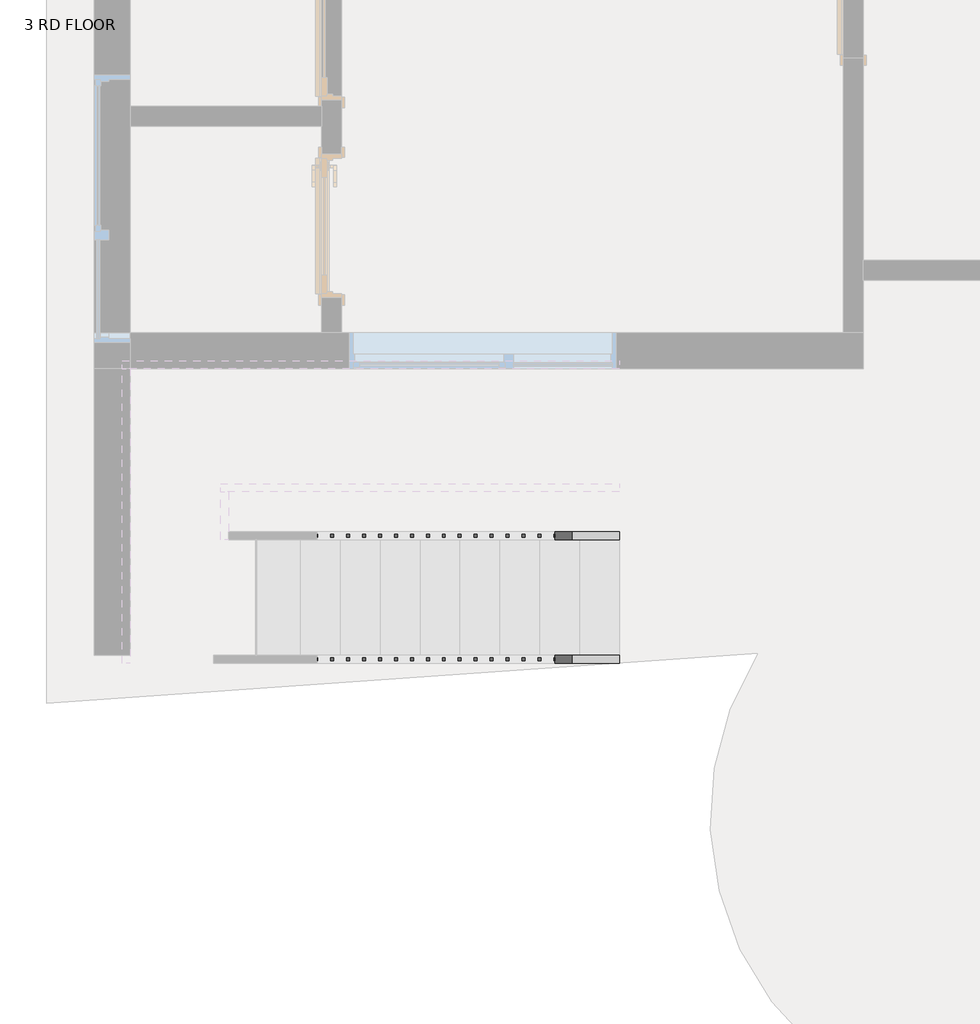
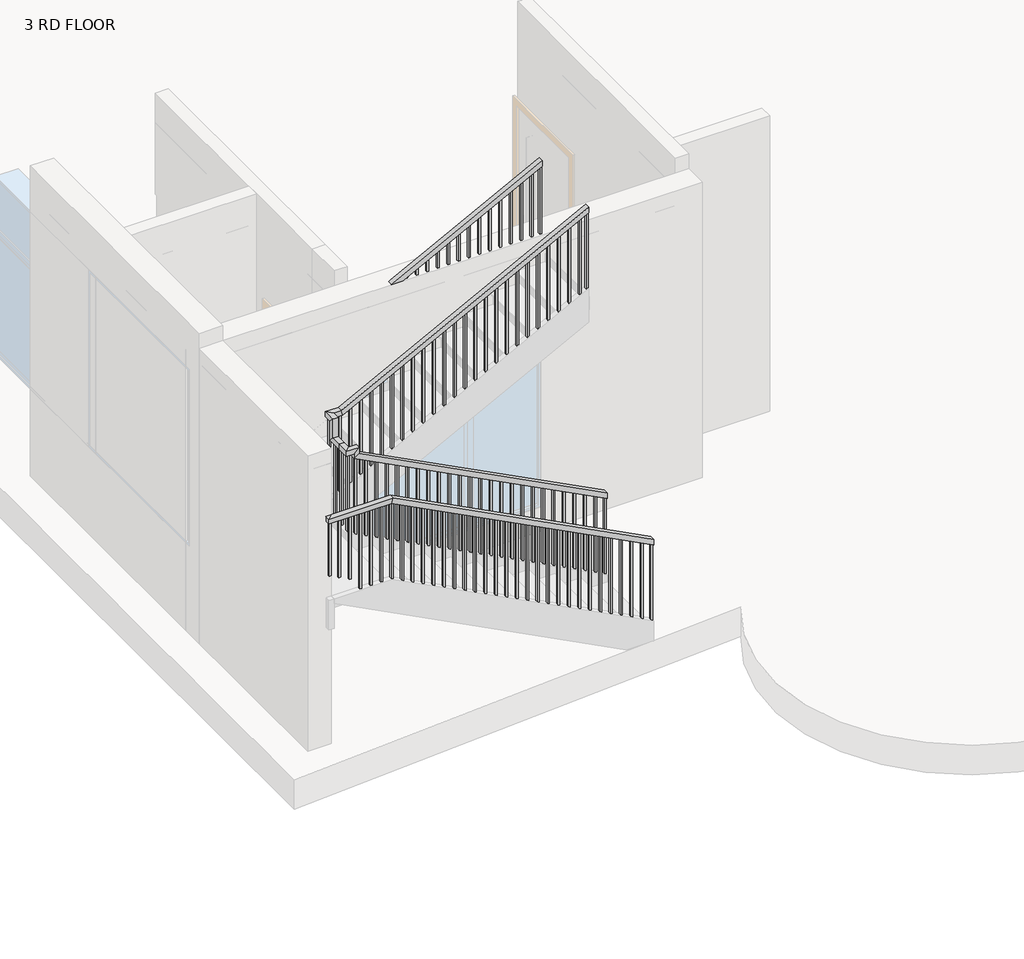
# One storey, part 4 of 5: 2 railings.
"""IFC4 building model written with IfcOpenShell, lengths in millimetres."""

from ifc_helpers import new_model, si_unit, frame, origin, place, context, project, spatial, polyline, outline, extrude, faceted_brep, element, save

model = new_model("IFC4")

# Units and contexts
model_context = context("Model", 3, world=origin())
ifc_project = project(units=[si_unit("LENGTHUNIT", "METRE", prefix="MILLI")], contexts=[model_context])

# Site, building, storey
site = spatial("IfcSite", under=ifc_project)
building = spatial("IfcBuilding", under=site)
storey = spatial("IfcBuildingStorey", under=building, Name="3 RD FLOOR", Elevation=9601.2)

# Railings
placement = place(None, origin())
element("IfcRailing", 1, ObjectType="Handrail - Rectangular", at=placement, inside=storey, context=model_context, shape_type="SolidModel", body=[
    faceted_brep([(-3117.2664982, -6914.3822004, 10647.2181818), (-3117.2664982, -6914.3822004, 10590.003028), (-3117.2664982, -6863.5822004, 10590.003028), (-3117.2664982, -6863.5822004, 10647.2181818), (-5530.2664982, -6914.3822004, 11897.5909091), (-5581.0664982, -6914.3822004, 11866.6993916), (-5581.0664982, -6863.5822004, 11866.6993916), (-5530.2664982, -6863.5822004, 11897.5909091), (-5657.2664982, -6787.3822004, 11912.6), (-5657.2664982, -6787.3822004, 11963.4), (-5657.2664982, -6685.7822004, 11963.4), (-5657.2664982, -6634.9822004, 11912.6), (-5606.4664982, -6787.3822004, 11912.6), (-5606.4664982, -6634.9822004, 11912.6), (-5606.4664982, -6787.3822004, 11963.4), (-5606.4664982, -6685.7822004, 11963.4), (-3117.2664982, -6558.7822004, 13411.2), (-3117.2664982, -6609.5822004, 13411.2), (-3117.2664982, -6609.5822004, 13353.9848461), (-3117.2664982, -6558.7822004, 13353.9848461), (-5517.8863767, -6558.7822004, 12110.0272727), (-5530.2664982, -6558.7822004, 12160.8272727), (-5517.8863767, -6609.5822004, 12110.0272727), (-5530.2664982, -6609.5822004, 12160.8272727), (-5530.2664982, -6914.3822004, 11963.4), (-5581.0664982, -6914.3822004, 11912.6), (-5581.0664982, -6863.5822004, 11912.6), (-5530.2664982, -6863.5822004, 11963.4), (-5657.2664982, -6914.3822004, 11963.4), (-5657.2664982, -6914.3822004, 11912.6), (-5606.4664982, -6863.5822004, 11912.6), (-5606.4664982, -6863.5822004, 11963.4), (-5657.2664982, -6685.7822004, 12160.8272727), (-5657.2664982, -6634.9822004, 12110.0272727), (-5606.4664982, -6634.9822004, 12110.0272727), (-5606.4664982, -6685.7822004, 12160.8272727), (-5657.2664982, -6558.7822004, 12160.8272727), (-5657.2664982, -6558.7822004, 12110.0272727), (-5606.4664982, -6609.5822004, 12110.0272727), (-5606.4664982, -6609.5822004, 12160.8272727)], [[[0, 1, 2, 3]], [[1, 0, 4, 5]], [[2, 1, 5, 6]], [[3, 2, 6, 7]], [[0, 3, 7, 4]], [[8, 9, 10, 11]], [[12, 8, 11, 13]], [[14, 12, 13, 15]], [[9, 14, 15, 10]], [[16, 17, 18, 19]], [[20, 21, 16, 19]], [[22, 20, 19, 18]], [[23, 22, 18, 17]], [[21, 23, 17, 16]], [[5, 4, 24, 25]], [[6, 5, 25, 26]], [[7, 6, 26, 27]], [[4, 7, 27, 24]], [[25, 24, 28, 29]], [[26, 25, 29, 30]], [[27, 26, 30, 31]], [[24, 27, 31, 28]], [[29, 28, 9, 8]], [[30, 29, 8, 12]], [[31, 30, 12, 14]], [[28, 31, 14, 9]], [[11, 10, 32, 33]], [[13, 11, 33, 34]], [[15, 13, 34, 35]], [[10, 15, 35, 32]], [[33, 32, 36, 37]], [[34, 33, 37, 38]], [[35, 34, 38, 39]], [[32, 35, 39, 36]], [[37, 36, 21, 20]], [[38, 37, 20, 22]], [[39, 38, 22, 23]], [[36, 39, 23, 21]]]),
    extrude(outline(polyline([(13319.4350734, -3183.9414982), (13309.5637098, -3202.9914982), (12525.2803899, -3202.9914982), (12535.1517536, -3183.9414982), (13319.4350734, -3183.9414982)])), frame((0.0, -6593.7072004, 0.0), z_axis=(0.0, 1.0, 0.0), x_axis=(0.0, 0.0, 1.0)), (0.0, 0.0, 1.0), 19.05),
    extrude(outline(polyline([(13266.7878007, -3285.5414982), (13256.916437, -3304.5914982), (12472.6331172, -3304.5914982), (12482.5044808, -3285.5414982), (13266.7878007, -3285.5414982)])), frame((0.0, -6593.7072004, 0.0), z_axis=(0.0, 1.0, 0.0), x_axis=(0.0, 0.0, 1.0)), (0.0, 0.0, 1.0), 19.05),
    extrude(outline(polyline([(13214.140528, -3387.1414982), (13204.2691643, -3406.1914982), (12419.9858445, -3406.1914982), (12429.8572081, -3387.1414982), (13214.140528, -3387.1414982)])), frame((0.0, -6593.7072004, 0.0), z_axis=(0.0, 1.0, 0.0), x_axis=(0.0, 0.0, 1.0)), (0.0, 0.0, 1.0), 19.05),
    extrude(outline(polyline([(13161.4932552, -3488.7414982), (13151.6218916, -3507.7914982), (12367.3385718, -3507.7914982), (12377.2099354, -3488.7414982), (13161.4932552, -3488.7414982)])), frame((0.0, -6593.7072004, 0.0), z_axis=(0.0, 1.0, 0.0), x_axis=(0.0, 0.0, 1.0)), (0.0, 0.0, 1.0), 19.05),
    extrude(outline(polyline([(13108.8459825, -3590.3414982), (13098.9746189, -3609.3914982), (12314.691299, -3609.3914982), (12324.5626627, -3590.3414982), (13108.8459825, -3590.3414982)])), frame((0.0, -6593.7072004, 0.0), z_axis=(0.0, 1.0, 0.0), x_axis=(0.0, 0.0, 1.0)), (0.0, 0.0, 1.0), 19.05),
    extrude(outline(polyline([(13056.1987098, -3691.9414982), (13046.3273461, -3710.9914982), (12262.0440263, -3710.9914982), (12271.9153899, -3691.9414982), (13056.1987098, -3691.9414982)])), frame((0.0, -6593.7072004, 0.0), z_axis=(0.0, 1.0, 0.0), x_axis=(0.0, 0.0, 1.0)), (0.0, 0.0, 1.0), 19.05),
    extrude(outline(polyline([(13003.551437, -3793.5414982), (12993.6800734, -3812.5914982), (12209.3967536, -3812.5914982), (12219.2681172, -3793.5414982), (13003.551437, -3793.5414982)])), frame((0.0, -6593.7072004, 0.0), z_axis=(0.0, 1.0, 0.0), x_axis=(0.0, 0.0, 1.0)), (0.0, 0.0, 1.0), 19.05),
    extrude(outline(polyline([(12950.9041643, -3895.1414982), (12941.0328007, -3914.1914982), (12156.7494808, -3914.1914982), (12166.6208445, -3895.1414982), (12950.9041643, -3895.1414982)])), frame((0.0, -6593.7072004, 0.0), z_axis=(0.0, 1.0, 0.0), x_axis=(0.0, 0.0, 1.0)), (0.0, 0.0, 1.0), 19.05),
    extrude(outline(polyline([(12898.2568916, -3996.7414982), (12888.385528, -4015.7914982), (12104.1022081, -4015.7914982), (12113.9735718, -3996.7414982), (12898.2568916, -3996.7414982)])), frame((0.0, -6593.7072004, 0.0), z_axis=(0.0, 1.0, 0.0), x_axis=(0.0, 0.0, 1.0)), (0.0, 0.0, 1.0), 19.05),
    extrude(outline(polyline([(12845.6096189, -4098.3414982), (12835.7382552, -4117.3914982), (12051.4549354, -4117.3914982), (12061.326299, -4098.3414982), (12845.6096189, -4098.3414982)])), frame((0.0, -6593.7072004, 0.0), z_axis=(0.0, 1.0, 0.0), x_axis=(0.0, 0.0, 1.0)), (0.0, 0.0, 1.0), 19.05),
    extrude(outline(polyline([(12792.9623461, -4199.9414982), (12783.0909825, -4218.9914982), (11998.8076627, -4218.9914982), (12008.6790263, -4199.9414982), (12792.9623461, -4199.9414982)])), frame((0.0, -6593.7072004, 0.0), z_axis=(0.0, 1.0, 0.0), x_axis=(0.0, 0.0, 1.0)), (0.0, 0.0, 1.0), 19.05),
    extrude(outline(polyline([(12740.3150734, -4301.5414982), (12730.4437098, -4320.5914982), (11946.1603899, -4320.5914982), (11956.0317536, -4301.5414982), (12740.3150734, -4301.5414982)])), frame((0.0, -6593.7072004, 0.0), z_axis=(0.0, 1.0, 0.0), x_axis=(0.0, 0.0, 1.0)), (0.0, 0.0, 1.0), 19.05),
    extrude(outline(polyline([(12687.6678007, -4403.1414982), (12677.796437, -4422.1914982), (11893.5131172, -4422.1914982), (11903.3844808, -4403.1414982), (12687.6678007, -4403.1414982)])), frame((0.0, -6593.7072004, 0.0), z_axis=(0.0, 1.0, 0.0), x_axis=(0.0, 0.0, 1.0)), (0.0, 0.0, 1.0), 19.05),
    extrude(outline(polyline([(12635.020528, -4504.7414982), (12625.1491643, -4523.7914982), (11840.8658445, -4523.7914982), (11850.7372081, -4504.7414982), (12635.020528, -4504.7414982)])), frame((0.0, -6593.7072004, 0.0), z_axis=(0.0, 1.0, 0.0), x_axis=(0.0, 0.0, 1.0)), (0.0, 0.0, 1.0), 19.05),
    extrude(outline(polyline([(12582.3732552, -4606.3414982), (12572.5018916, -4625.3914982), (11788.2185718, -4625.3914982), (11798.0899354, -4606.3414982), (12582.3732552, -4606.3414982)])), frame((0.0, -6593.7072004, 0.0), z_axis=(0.0, 1.0, 0.0), x_axis=(0.0, 0.0, 1.0)), (0.0, 0.0, 1.0), 19.05),
    extrude(outline(polyline([(12529.7259825, -4707.9414982), (12519.8546189, -4726.9914982), (11735.571299, -4726.9914982), (11745.4426627, -4707.9414982), (12529.7259825, -4707.9414982)])), frame((0.0, -6593.7072004, 0.0), z_axis=(0.0, 1.0, 0.0), x_axis=(0.0, 0.0, 1.0)), (0.0, 0.0, 1.0), 19.05),
    extrude(outline(polyline([(12477.0787098, -4809.5414982), (12467.2073461, -4828.5914982), (11682.9240263, -4828.5914982), (11692.7953899, -4809.5414982), (12477.0787098, -4809.5414982)])), frame((0.0, -6593.7072004, 0.0), z_axis=(0.0, 1.0, 0.0), x_axis=(0.0, 0.0, 1.0)), (0.0, 0.0, 1.0), 19.05),
    extrude(outline(polyline([(12424.431437, -4911.1414982), (12414.5600734, -4930.1914982), (11630.2767536, -4930.1914982), (11640.1481172, -4911.1414982), (12424.431437, -4911.1414982)])), frame((0.0, -6593.7072004, 0.0), z_axis=(0.0, 1.0, 0.0), x_axis=(0.0, 0.0, 1.0)), (0.0, 0.0, 1.0), 19.05),
    extrude(outline(polyline([(12371.7841643, -5012.7414982), (12361.9128007, -5031.7914982), (11577.6294808, -5031.7914982), (11587.5008445, -5012.7414982), (12371.7841643, -5012.7414982)])), frame((0.0, -6593.7072004, 0.0), z_axis=(0.0, 1.0, 0.0), x_axis=(0.0, 0.0, 1.0)), (0.0, 0.0, 1.0), 19.05),
    extrude(outline(polyline([(12319.1368916, -5114.3414982), (12309.265528, -5133.3914982), (11524.9822081, -5133.3914982), (11534.8535718, -5114.3414982), (12319.1368916, -5114.3414982)])), frame((0.0, -6593.7072004, 0.0), z_axis=(0.0, 1.0, 0.0), x_axis=(0.0, 0.0, 1.0)), (0.0, 0.0, 1.0), 19.05),
    extrude(outline(polyline([(12266.4896189, -5215.9414982), (12256.6182552, -5234.9914982), (11472.3349354, -5234.9914982), (11482.206299, -5215.9414982), (12266.4896189, -5215.9414982)])), frame((0.0, -6593.7072004, 0.0), z_axis=(0.0, 1.0, 0.0), x_axis=(0.0, 0.0, 1.0)), (0.0, 0.0, 1.0), 19.05),
    extrude(outline(polyline([(12213.8423461, -5317.5414982), (12203.9709825, -5336.5914982), (11419.6876627, -5336.5914982), (11429.5590263, -5317.5414982), (12213.8423461, -5317.5414982)])), frame((0.0, -6593.7072004, 0.0), z_axis=(0.0, 1.0, 0.0), x_axis=(0.0, 0.0, 1.0)), (0.0, 0.0, 1.0), 19.05),
    extrude(outline(polyline([(12161.1950734, -5419.1414982), (12151.3237098, -5438.1914982), (11367.0403899, -5438.1914982), (11376.9117536, -5419.1414982), (12161.1950734, -5419.1414982)])), frame((0.0, -6593.7072004, 0.0), z_axis=(0.0, 1.0, 0.0), x_axis=(0.0, 0.0, 1.0)), (0.0, 0.0, 1.0), 19.05),
    extrude(outline(polyline([(12108.5478007, -5520.7414982), (12098.676437, -5539.7914982), (11314.3931172, -5539.7914982), (11324.2644808, -5520.7414982), (12108.5478007, -5520.7414982)])), frame((0.0, -6593.7072004, 0.0), z_axis=(0.0, 1.0, 0.0), x_axis=(0.0, 0.0, 1.0)), (0.0, 0.0, 1.0), 19.05),
    extrude(outline(polyline([(-5622.3414982, -6695.3072004), (-5641.3914982, -6695.3072004), (-5641.3914982, -6676.2572004), (-5622.3414982, -6676.2572004), (-5622.3414982, -6695.3072004)])), frame((0.0, 0.0, 11125.2), z_axis=(0.0, 0.0, 1.0), x_axis=(1.0, 0.0, 0.0)), (0.0, 0.0, 1.0), 787.4),
    extrude(outline(polyline([(-5622.3414982, -6796.9072004), (-5641.3914982, -6796.9072004), (-5641.3914982, -6777.8572004), (-5622.3414982, -6777.8572004), (-5622.3414982, -6796.9072004)])), frame((0.0, 0.0, 11125.2), z_axis=(0.0, 0.0, 1.0), x_axis=(1.0, 0.0, 0.0)), (0.0, 0.0, 1.0), 787.4),
    extrude(outline(polyline([(11912.6, -5546.1414982), (11912.6, -5565.1914982), (11074.1899354, -5565.1914982), (11064.3185718, -5546.1414982), (11912.6, -5546.1414982)])), frame((0.0, -6898.5072004, 0.0), z_axis=(0.0, 1.0, 0.0), x_axis=(0.0, 0.0, 1.0)), (0.0, 0.0, 1.0), 19.05),
    extrude(outline(polyline([(11795.9546189, -5444.5414982), (11805.8259825, -5463.5914982), (11021.5426627, -5463.5914982), (11011.671299, -5444.5414982), (11795.9546189, -5444.5414982)])), frame((0.0, -6898.5072004, 0.0), z_axis=(0.0, 1.0, 0.0), x_axis=(0.0, 0.0, 1.0)), (0.0, 0.0, 1.0), 19.05),
    extrude(outline(polyline([(11743.3073461, -5342.9414982), (11753.1787098, -5361.9914982), (10968.8953899, -5361.9914982), (10959.0240263, -5342.9414982), (11743.3073461, -5342.9414982)])), frame((0.0, -6898.5072004, 0.0), z_axis=(0.0, 1.0, 0.0), x_axis=(0.0, 0.0, 1.0)), (0.0, 0.0, 1.0), 19.05),
    extrude(outline(polyline([(11690.6600734, -5241.3414982), (11700.531437, -5260.3914982), (10916.2481172, -5260.3914982), (10906.3767536, -5241.3414982), (11690.6600734, -5241.3414982)])), frame((0.0, -6898.5072004, 0.0), z_axis=(0.0, 1.0, 0.0), x_axis=(0.0, 0.0, 1.0)), (0.0, 0.0, 1.0), 19.05),
    extrude(outline(polyline([(11638.0128007, -5139.7414982), (11647.8841643, -5158.7914982), (10863.6008445, -5158.7914982), (10853.7294808, -5139.7414982), (11638.0128007, -5139.7414982)])), frame((0.0, -6898.5072004, 0.0), z_axis=(0.0, 1.0, 0.0), x_axis=(0.0, 0.0, 1.0)), (0.0, 0.0, 1.0), 19.05),
    extrude(outline(polyline([(11585.365528, -5038.1414982), (11595.2368916, -5057.1914982), (10810.9535718, -5057.1914982), (10801.0822081, -5038.1414982), (11585.365528, -5038.1414982)])), frame((0.0, -6898.5072004, 0.0), z_axis=(0.0, 1.0, 0.0), x_axis=(0.0, 0.0, 1.0)), (0.0, 0.0, 1.0), 19.05),
    extrude(outline(polyline([(11532.7182552, -4936.5414982), (11542.5896189, -4955.5914982), (10758.306299, -4955.5914982), (10748.4349354, -4936.5414982), (11532.7182552, -4936.5414982)])), frame((0.0, -6898.5072004, 0.0), z_axis=(0.0, 1.0, 0.0), x_axis=(0.0, 0.0, 1.0)), (0.0, 0.0, 1.0), 19.05),
    extrude(outline(polyline([(11480.0709825, -4834.9414982), (11489.9423461, -4853.9914982), (10705.6590263, -4853.9914982), (10695.7876627, -4834.9414982), (11480.0709825, -4834.9414982)])), frame((0.0, -6898.5072004, 0.0), z_axis=(0.0, 1.0, 0.0), x_axis=(0.0, 0.0, 1.0)), (0.0, 0.0, 1.0), 19.05),
    extrude(outline(polyline([(11427.4237098, -4733.3414982), (11437.2950734, -4752.3914982), (10653.0117536, -4752.3914982), (10643.1403899, -4733.3414982), (11427.4237098, -4733.3414982)])), frame((0.0, -6898.5072004, 0.0), z_axis=(0.0, 1.0, 0.0), x_axis=(0.0, 0.0, 1.0)), (0.0, 0.0, 1.0), 19.05),
    extrude(outline(polyline([(11374.776437, -4631.7414982), (11384.6478007, -4650.7914982), (10600.3644808, -4650.7914982), (10590.4931172, -4631.7414982), (11374.776437, -4631.7414982)])), frame((0.0, -6898.5072004, 0.0), z_axis=(0.0, 1.0, 0.0), x_axis=(0.0, 0.0, 1.0)), (0.0, 0.0, 1.0), 19.05),
    extrude(outline(polyline([(11322.1291643, -4530.1414982), (11332.000528, -4549.1914982), (10547.7172081, -4549.1914982), (10537.8458445, -4530.1414982), (11322.1291643, -4530.1414982)])), frame((0.0, -6898.5072004, 0.0), z_axis=(0.0, 1.0, 0.0), x_axis=(0.0, 0.0, 1.0)), (0.0, 0.0, 1.0), 19.05),
    extrude(outline(polyline([(11269.4818916, -4428.5414982), (11279.3532552, -4447.5914982), (10495.0699354, -4447.5914982), (10485.1985718, -4428.5414982), (11269.4818916, -4428.5414982)])), frame((0.0, -6898.5072004, 0.0), z_axis=(0.0, 1.0, 0.0), x_axis=(0.0, 0.0, 1.0)), (0.0, 0.0, 1.0), 19.05),
    extrude(outline(polyline([(11216.8346189, -4326.9414982), (11226.7059825, -4345.9914982), (10442.4226627, -4345.9914982), (10432.551299, -4326.9414982), (11216.8346189, -4326.9414982)])), frame((0.0, -6898.5072004, 0.0), z_axis=(0.0, 1.0, 0.0), x_axis=(0.0, 0.0, 1.0)), (0.0, 0.0, 1.0), 19.05),
    extrude(outline(polyline([(11164.1873461, -4225.3414982), (11174.0587098, -4244.3914982), (10389.7753899, -4244.3914982), (10379.9040263, -4225.3414982), (11164.1873461, -4225.3414982)])), frame((0.0, -6898.5072004, 0.0), z_axis=(0.0, 1.0, 0.0), x_axis=(0.0, 0.0, 1.0)), (0.0, 0.0, 1.0), 19.05),
    extrude(outline(polyline([(11111.5400734, -4123.7414982), (11121.411437, -4142.7914982), (10337.1281172, -4142.7914982), (10327.2567536, -4123.7414982), (11111.5400734, -4123.7414982)])), frame((0.0, -6898.5072004, 0.0), z_axis=(0.0, 1.0, 0.0), x_axis=(0.0, 0.0, 1.0)), (0.0, 0.0, 1.0), 19.05),
    extrude(outline(polyline([(11058.8928007, -4022.1414982), (11068.7641643, -4041.1914982), (10284.4808445, -4041.1914982), (10274.6094808, -4022.1414982), (11058.8928007, -4022.1414982)])), frame((0.0, -6898.5072004, 0.0), z_axis=(0.0, 1.0, 0.0), x_axis=(0.0, 0.0, 1.0)), (0.0, 0.0, 1.0), 19.05),
    extrude(outline(polyline([(11006.245528, -3920.5414982), (11016.1168916, -3939.5914982), (10231.8335718, -3939.5914982), (10221.9622081, -3920.5414982), (11006.245528, -3920.5414982)])), frame((0.0, -6898.5072004, 0.0), z_axis=(0.0, 1.0, 0.0), x_axis=(0.0, 0.0, 1.0)), (0.0, 0.0, 1.0), 19.05),
    extrude(outline(polyline([(10953.5982552, -3818.9414982), (10963.4696189, -3837.9914982), (10179.186299, -3837.9914982), (10169.3149354, -3818.9414982), (10953.5982552, -3818.9414982)])), frame((0.0, -6898.5072004, 0.0), z_axis=(0.0, 1.0, 0.0), x_axis=(0.0, 0.0, 1.0)), (0.0, 0.0, 1.0), 19.05),
    extrude(outline(polyline([(10900.9509825, -3717.3414982), (10910.8223461, -3736.3914982), (10126.5390263, -3736.3914982), (10116.6676627, -3717.3414982), (10900.9509825, -3717.3414982)])), frame((0.0, -6898.5072004, 0.0), z_axis=(0.0, 1.0, 0.0), x_axis=(0.0, 0.0, 1.0)), (0.0, 0.0, 1.0), 19.05),
    extrude(outline(polyline([(10848.3037098, -3615.7414982), (10858.1750734, -3634.7914982), (10073.8917536, -3634.7914982), (10064.0203899, -3615.7414982), (10848.3037098, -3615.7414982)])), frame((0.0, -6898.5072004, 0.0), z_axis=(0.0, 1.0, 0.0), x_axis=(0.0, 0.0, 1.0)), (0.0, 0.0, 1.0), 19.05),
    extrude(outline(polyline([(10795.656437, -3514.1414982), (10805.5278007, -3533.1914982), (10021.2444808, -3533.1914982), (10011.3731172, -3514.1414982), (10795.656437, -3514.1414982)])), frame((0.0, -6898.5072004, 0.0), z_axis=(0.0, 1.0, 0.0), x_axis=(0.0, 0.0, 1.0)), (0.0, 0.0, 1.0), 19.05),
    extrude(outline(polyline([(10743.0091643, -3412.5414982), (10752.880528, -3431.5914982), (9968.5972081, -3431.5914982), (9958.7258445, -3412.5414982), (10743.0091643, -3412.5414982)])), frame((0.0, -6898.5072004, 0.0), z_axis=(0.0, 1.0, 0.0), x_axis=(0.0, 0.0, 1.0)), (0.0, 0.0, 1.0), 19.05),
    extrude(outline(polyline([(10690.3618916, -3310.9414982), (10700.2332552, -3329.9914982), (9915.9499354, -3329.9914982), (9906.0785718, -3310.9414982), (10690.3618916, -3310.9414982)])), frame((0.0, -6898.5072004, 0.0), z_axis=(0.0, 1.0, 0.0), x_axis=(0.0, 0.0, 1.0)), (0.0, 0.0, 1.0), 19.05),
    extrude(outline(polyline([(10637.7146189, -3209.3414982), (10647.5859825, -3228.3914982), (9863.3026627, -3228.3914982), (9853.431299, -3209.3414982), (10637.7146189, -3209.3414982)])), frame((0.0, -6898.5072004, 0.0), z_axis=(0.0, 1.0, 0.0), x_axis=(0.0, 0.0, 1.0)), (0.0, 0.0, 1.0), 19.05),
    extrude(outline(polyline([(-6593.7072004, 12110.0272727), (-6574.6572004, 12110.0272727), (-6574.6572004, 11271.6172081), (-6593.7072004, 11261.7458445), (-6593.7072004, 12110.0272727)])), frame((-5641.3914982, 0.0, 0.0), z_axis=(1.0, 0.0, 0.0), x_axis=(0.0, 1.0, 0.0)), (0.0, 0.0, 1.0), 19.05),
    extrude(outline(polyline([(-5622.3414982, -6879.4572004), (-5622.3414982, -6898.5072004), (-5641.3914982, -6898.5072004), (-5641.3914982, -6879.4572004), (-5622.3414982, -6879.4572004)])), frame((0.0, 0.0, 11125.2), z_axis=(0.0, 0.0, 1.0), x_axis=(1.0, 0.0, 0.0)), (0.0, 0.0, 1.0), 787.4),
    extrude(outline(polyline([(13353.9848461, -3117.2664982), (13344.1134825, -3136.3164982), (12559.8301627, -3136.3164982), (12569.7015263, -3117.2664982), (13353.9848461, -3117.2664982)])), frame((0.0, -6593.7072004, 0.0), z_axis=(0.0, 1.0, 0.0), x_axis=(0.0, 0.0, 1.0)), (0.0, 0.0, 1.0), 19.05),
    extrude(outline(polyline([(10590.003028, -3117.2664982), (10599.8743916, -3136.3164982), (9815.5910718, -3136.3164982), (9805.7197081, -3117.2664982), (10590.003028, -3117.2664982)])), frame((0.0, -6898.5072004, 0.0), z_axis=(0.0, 1.0, 0.0), x_axis=(0.0, 0.0, 1.0)), (0.0, 0.0, 1.0), 19.05),
])
element("IfcRailing", 2, ObjectType="Handrail - Rectangular", at=placement, inside=storey, context=model_context, shape_type="SolidModel", body=[
    faceted_brep([(-3117.2664982, -7701.7822004, 10647.2181818), (-3117.2664982, -7701.7822004, 10590.003028), (-3117.2664982, -7650.9822004, 10590.003028), (-3117.2664982, -7650.9822004, 10647.2181818), (-5657.2664982, -7701.7822004, 11963.4), (-5669.6466197, -7701.7822004, 11912.6), (-5669.6466197, -7650.9822004, 11912.6), (-5657.2664982, -7650.9822004, 11963.4), (-6283.3131972, -7701.7822004, 11912.6), (-6283.3131972, -7701.7822004, 11963.4), (-6283.3131972, -5773.9082131, 11963.4), (-6283.3131972, -5773.9082131, 11912.6), (-6232.5131972, -7650.9822004, 11912.6), (-6232.5131972, -5824.7082131, 11912.6), (-6232.5131972, -7650.9822004, 11963.4), (-6232.5131972, -5824.7082131, 11963.4), (-5911.2664982, -5773.9082131, 11963.4), (-5898.8863767, -5773.9082131, 11912.6), (-5898.8863767, -5824.7082131, 11912.6), (-5911.2664982, -5824.7082131, 11963.4), (-3117.2664982, -5773.9082131, 13411.2), (-3117.2664982, -5824.7082131, 13411.2), (-3117.2664982, -5824.7082131, 13353.9848461), (-3117.2664982, -5773.9082131, 13353.9848461)], [[[0, 1, 2, 3]], [[1, 0, 4, 5]], [[2, 1, 5, 6]], [[3, 2, 6, 7]], [[0, 3, 7, 4]], [[8, 9, 10, 11]], [[12, 8, 11, 13]], [[14, 12, 13, 15]], [[9, 14, 15, 10]], [[11, 10, 16, 17]], [[13, 11, 17, 18]], [[15, 13, 18, 19]], [[10, 15, 19, 16]], [[5, 4, 9, 8]], [[6, 5, 8, 12]], [[7, 6, 12, 14]], [[4, 7, 14, 9]], [[20, 21, 22, 23]], [[17, 16, 20, 23]], [[18, 17, 23, 22]], [[19, 18, 22, 21]], [[16, 19, 21, 20]]]),
    extrude(outline(polyline([(13301.0413294, -3219.4381972), (12516.7580095, -3219.4381972), (12526.6293732, -3200.3881972), (13310.912693, -3200.3881972), (13301.0413294, -3219.4381972)])), frame((0.0, -5808.8332131, 0.0), z_axis=(0.0, 1.0, 0.0), x_axis=(0.0, 0.0, 1.0)), (0.0, 0.0, 1.0), 19.05),
    extrude(outline(polyline([(13248.3940566, -3321.0381972), (12464.1107368, -3321.0381972), (12473.9821004, -3301.9881972), (13258.2654203, -3301.9881972), (13248.3940566, -3321.0381972)])), frame((0.0, -5808.8332131, 0.0), z_axis=(0.0, 1.0, 0.0), x_axis=(0.0, 0.0, 1.0)), (0.0, 0.0, 1.0), 19.05),
    extrude(outline(polyline([(13195.7467839, -3422.6381972), (12411.4634641, -3422.6381972), (12421.3348277, -3403.5881972), (13205.6181476, -3403.5881972), (13195.7467839, -3422.6381972)])), frame((0.0, -5808.8332131, 0.0), z_axis=(0.0, 1.0, 0.0), x_axis=(0.0, 0.0, 1.0)), (0.0, 0.0, 1.0), 19.05),
    extrude(outline(polyline([(13143.0995112, -3524.2381972), (12358.8161913, -3524.2381972), (12368.687555, -3505.1881972), (13152.9708748, -3505.1881972), (13143.0995112, -3524.2381972)])), frame((0.0, -5808.8332131, 0.0), z_axis=(0.0, 1.0, 0.0), x_axis=(0.0, 0.0, 1.0)), (0.0, 0.0, 1.0), 19.05),
    extrude(outline(polyline([(13090.4522385, -3625.8381972), (12306.1689186, -3625.8381972), (12316.0402823, -3606.7881972), (13100.3236021, -3606.7881972), (13090.4522385, -3625.8381972)])), frame((0.0, -5808.8332131, 0.0), z_axis=(0.0, 1.0, 0.0), x_axis=(0.0, 0.0, 1.0)), (0.0, 0.0, 1.0), 19.05),
    extrude(outline(polyline([(13037.8049657, -3727.4381972), (12253.5216459, -3727.4381972), (12263.3930095, -3708.3881972), (13047.6763294, -3708.3881972), (13037.8049657, -3727.4381972)])), frame((0.0, -5808.8332131, 0.0), z_axis=(0.0, 1.0, 0.0), x_axis=(0.0, 0.0, 1.0)), (0.0, 0.0, 1.0), 19.05),
    extrude(outline(polyline([(12985.157693, -3829.0381972), (12200.8743732, -3829.0381972), (12210.7457368, -3809.9881972), (12995.0290566, -3809.9881972), (12985.157693, -3829.0381972)])), frame((0.0, -5808.8332131, 0.0), z_axis=(0.0, 1.0, 0.0), x_axis=(0.0, 0.0, 1.0)), (0.0, 0.0, 1.0), 19.05),
    extrude(outline(polyline([(12932.5104203, -3930.6381972), (12148.2271004, -3930.6381972), (12158.0984641, -3911.5881972), (12942.3817839, -3911.5881972), (12932.5104203, -3930.6381972)])), frame((0.0, -5808.8332131, 0.0), z_axis=(0.0, 1.0, 0.0), x_axis=(0.0, 0.0, 1.0)), (0.0, 0.0, 1.0), 19.05),
    extrude(outline(polyline([(12879.8631476, -4032.2381972), (12095.5798277, -4032.2381972), (12105.4511913, -4013.1881972), (12889.7345112, -4013.1881972), (12879.8631476, -4032.2381972)])), frame((0.0, -5808.8332131, 0.0), z_axis=(0.0, 1.0, 0.0), x_axis=(0.0, 0.0, 1.0)), (0.0, 0.0, 1.0), 19.05),
    extrude(outline(polyline([(12827.2158748, -4133.8381972), (12042.932555, -4133.8381972), (12052.8039186, -4114.7881972), (12837.0872385, -4114.7881972), (12827.2158748, -4133.8381972)])), frame((0.0, -5808.8332131, 0.0), z_axis=(0.0, 1.0, 0.0), x_axis=(0.0, 0.0, 1.0)), (0.0, 0.0, 1.0), 19.05),
    extrude(outline(polyline([(12774.5686021, -4235.4381972), (11990.2852823, -4235.4381972), (12000.1566459, -4216.3881972), (12784.4399657, -4216.3881972), (12774.5686021, -4235.4381972)])), frame((0.0, -5808.8332131, 0.0), z_axis=(0.0, 1.0, 0.0), x_axis=(0.0, 0.0, 1.0)), (0.0, 0.0, 1.0), 19.05),
    extrude(outline(polyline([(12721.9213294, -4337.0381972), (11937.6380095, -4337.0381972), (11947.5093732, -4317.9881972), (12731.792693, -4317.9881972), (12721.9213294, -4337.0381972)])), frame((0.0, -5808.8332131, 0.0), z_axis=(0.0, 1.0, 0.0), x_axis=(0.0, 0.0, 1.0)), (0.0, 0.0, 1.0), 19.05),
    extrude(outline(polyline([(12669.2740566, -4438.6381972), (11884.9907368, -4438.6381972), (11894.8621004, -4419.5881972), (12679.1454203, -4419.5881972), (12669.2740566, -4438.6381972)])), frame((0.0, -5808.8332131, 0.0), z_axis=(0.0, 1.0, 0.0), x_axis=(0.0, 0.0, 1.0)), (0.0, 0.0, 1.0), 19.05),
    extrude(outline(polyline([(12616.6267839, -4540.2381972), (11832.3434641, -4540.2381972), (11842.2148277, -4521.1881972), (12626.4981476, -4521.1881972), (12616.6267839, -4540.2381972)])), frame((0.0, -5808.8332131, 0.0), z_axis=(0.0, 1.0, 0.0), x_axis=(0.0, 0.0, 1.0)), (0.0, 0.0, 1.0), 19.05),
    extrude(outline(polyline([(12563.9795112, -4641.8381972), (11779.6961913, -4641.8381972), (11789.567555, -4622.7881972), (12573.8508748, -4622.7881972), (12563.9795112, -4641.8381972)])), frame((0.0, -5808.8332131, 0.0), z_axis=(0.0, 1.0, 0.0), x_axis=(0.0, 0.0, 1.0)), (0.0, 0.0, 1.0), 19.05),
    extrude(outline(polyline([(12511.3322385, -4743.4381972), (11727.0489186, -4743.4381972), (11736.9202823, -4724.3881972), (12521.2036021, -4724.3881972), (12511.3322385, -4743.4381972)])), frame((0.0, -5808.8332131, 0.0), z_axis=(0.0, 1.0, 0.0), x_axis=(0.0, 0.0, 1.0)), (0.0, 0.0, 1.0), 19.05),
    extrude(outline(polyline([(12458.6849657, -4845.0381972), (11674.4016459, -4845.0381972), (11684.2730095, -4825.9881972), (12468.5563294, -4825.9881972), (12458.6849657, -4845.0381972)])), frame((0.0, -5808.8332131, 0.0), z_axis=(0.0, 1.0, 0.0), x_axis=(0.0, 0.0, 1.0)), (0.0, 0.0, 1.0), 19.05),
    extrude(outline(polyline([(12406.037693, -4946.6381972), (11621.7543732, -4946.6381972), (11631.6257368, -4927.5881972), (12415.9090566, -4927.5881972), (12406.037693, -4946.6381972)])), frame((0.0, -5808.8332131, 0.0), z_axis=(0.0, 1.0, 0.0), x_axis=(0.0, 0.0, 1.0)), (0.0, 0.0, 1.0), 19.05),
    extrude(outline(polyline([(12353.3904203, -5048.2381972), (11569.1071004, -5048.2381972), (11578.9784641, -5029.1881972), (12363.2617839, -5029.1881972), (12353.3904203, -5048.2381972)])), frame((0.0, -5808.8332131, 0.0), z_axis=(0.0, 1.0, 0.0), x_axis=(0.0, 0.0, 1.0)), (0.0, 0.0, 1.0), 19.05),
    extrude(outline(polyline([(12300.7431476, -5149.8381972), (11516.4598277, -5149.8381972), (11526.3311913, -5130.7881972), (12310.6145112, -5130.7881972), (12300.7431476, -5149.8381972)])), frame((0.0, -5808.8332131, 0.0), z_axis=(0.0, 1.0, 0.0), x_axis=(0.0, 0.0, 1.0)), (0.0, 0.0, 1.0), 19.05),
    extrude(outline(polyline([(12248.0958748, -5251.4381972), (11463.812555, -5251.4381972), (11473.6839186, -5232.3881972), (12257.9672385, -5232.3881972), (12248.0958748, -5251.4381972)])), frame((0.0, -5808.8332131, 0.0), z_axis=(0.0, 1.0, 0.0), x_axis=(0.0, 0.0, 1.0)), (0.0, 0.0, 1.0), 19.05),
    extrude(outline(polyline([(12195.4486021, -5353.0381972), (11411.1652823, -5353.0381972), (11421.0366459, -5333.9881972), (12205.3199657, -5333.9881972), (12195.4486021, -5353.0381972)])), frame((0.0, -5808.8332131, 0.0), z_axis=(0.0, 1.0, 0.0), x_axis=(0.0, 0.0, 1.0)), (0.0, 0.0, 1.0), 19.05),
    extrude(outline(polyline([(12142.8013294, -5454.6381972), (11358.5180095, -5454.6381972), (11368.3893732, -5435.5881972), (12152.672693, -5435.5881972), (12142.8013294, -5454.6381972)])), frame((0.0, -5808.8332131, 0.0), z_axis=(0.0, 1.0, 0.0), x_axis=(0.0, 0.0, 1.0)), (0.0, 0.0, 1.0), 19.05),
    extrude(outline(polyline([(12090.1540566, -5556.2381972), (11305.8707368, -5556.2381972), (11315.7421004, -5537.1881972), (12100.0254203, -5537.1881972), (12090.1540566, -5556.2381972)])), frame((0.0, -5808.8332131, 0.0), z_axis=(0.0, 1.0, 0.0), x_axis=(0.0, 0.0, 1.0)), (0.0, 0.0, 1.0), 19.05),
    extrude(outline(polyline([(12037.5067839, -5657.8381972), (11253.2234641, -5657.8381972), (11263.0948277, -5638.7881972), (12047.3781476, -5638.7881972), (12037.5067839, -5657.8381972)])), frame((0.0, -5808.8332131, 0.0), z_axis=(0.0, 1.0, 0.0), x_axis=(0.0, 0.0, 1.0)), (0.0, 0.0, 1.0), 19.05),
    extrude(outline(polyline([(11984.8595112, -5759.4381972), (11200.5761913, -5759.4381972), (11210.447555, -5740.3881972), (11994.7308748, -5740.3881972), (11984.8595112, -5759.4381972)])), frame((0.0, -5808.8332131, 0.0), z_axis=(0.0, 1.0, 0.0), x_axis=(0.0, 0.0, 1.0)), (0.0, 0.0, 1.0), 19.05),
    extrude(outline(polyline([(11932.2122385, -5861.0381972), (11147.9289186, -5861.0381972), (11157.8002823, -5841.9881972), (11942.0836021, -5841.9881972), (11932.2122385, -5861.0381972)])), frame((0.0, -5808.8332131, 0.0), z_axis=(0.0, 1.0, 0.0), x_axis=(0.0, 0.0, 1.0)), (0.0, 0.0, 1.0), 19.05),
    extrude(outline(polyline([(11912.6, -5962.6381972), (11095.2816459, -5962.6381972), (11105.1530095, -5943.5881972), (11912.6, -5943.5881972), (11912.6, -5962.6381972)])), frame((0.0, -5808.8332131, 0.0), z_axis=(0.0, 1.0, 0.0), x_axis=(0.0, 0.0, 1.0)), (0.0, 0.0, 1.0), 19.05),
    extrude(outline(polyline([(11912.6, -6064.2381972), (11042.6343732, -6064.2381972), (11052.5057368, -6045.1881972), (11912.6, -6045.1881972), (11912.6, -6064.2381972)])), frame((0.0, -5808.8332131, 0.0), z_axis=(0.0, 1.0, 0.0), x_axis=(0.0, 0.0, 1.0)), (0.0, 0.0, 1.0), 19.05),
    extrude(outline(polyline([(11912.6, -6165.8381972), (10989.9871004, -6165.8381972), (10999.8584641, -6146.7881972), (11912.6, -6146.7881972), (11912.6, -6165.8381972)])), frame((0.0, -5808.8332131, 0.0), z_axis=(0.0, 1.0, 0.0), x_axis=(0.0, 0.0, 1.0)), (0.0, 0.0, 1.0), 19.05),
    extrude(outline(polyline([(-6267.4381972, -5857.1072004), (-6267.4381972, -5838.0572004), (-6248.3881972, -5838.0572004), (-6248.3881972, -5857.1072004), (-6267.4381972, -5857.1072004)])), frame((0.0, 0.0, 11125.2), z_axis=(0.0, 0.0, 1.0), x_axis=(1.0, 0.0, 0.0)), (0.0, 0.0, 1.0), 787.4),
    extrude(outline(polyline([(-6267.4381972, -5958.7072004), (-6267.4381972, -5939.6572004), (-6248.3881972, -5939.6572004), (-6248.3881972, -5958.7072004), (-6267.4381972, -5958.7072004)])), frame((0.0, 0.0, 11125.2), z_axis=(0.0, 0.0, 1.0), x_axis=(1.0, 0.0, 0.0)), (0.0, 0.0, 1.0), 787.4),
    extrude(outline(polyline([(-6267.4381972, -6060.3072004), (-6267.4381972, -6041.2572004), (-6248.3881972, -6041.2572004), (-6248.3881972, -6060.3072004), (-6267.4381972, -6060.3072004)])), frame((0.0, 0.0, 11125.2), z_axis=(0.0, 0.0, 1.0), x_axis=(1.0, 0.0, 0.0)), (0.0, 0.0, 1.0), 787.4),
    extrude(outline(polyline([(-6267.4381972, -6161.9072004), (-6267.4381972, -6142.8572004), (-6248.3881972, -6142.8572004), (-6248.3881972, -6161.9072004), (-6267.4381972, -6161.9072004)])), frame((0.0, 0.0, 11125.2), z_axis=(0.0, 0.0, 1.0), x_axis=(1.0, 0.0, 0.0)), (0.0, 0.0, 1.0), 787.4),
    extrude(outline(polyline([(-6267.4381972, -6263.5072004), (-6267.4381972, -6244.4572004), (-6248.3881972, -6244.4572004), (-6248.3881972, -6263.5072004), (-6267.4381972, -6263.5072004)])), frame((0.0, 0.0, 11125.2), z_axis=(0.0, 0.0, 1.0), x_axis=(1.0, 0.0, 0.0)), (0.0, 0.0, 1.0), 787.4),
    extrude(outline(polyline([(-6267.4381972, -6365.1072004), (-6267.4381972, -6346.0572004), (-6248.3881972, -6346.0572004), (-6248.3881972, -6365.1072004), (-6267.4381972, -6365.1072004)])), frame((0.0, 0.0, 11125.2), z_axis=(0.0, 0.0, 1.0), x_axis=(1.0, 0.0, 0.0)), (0.0, 0.0, 1.0), 787.4),
    extrude(outline(polyline([(-6267.4381972, -6466.7072004), (-6267.4381972, -6447.6572004), (-6248.3881972, -6447.6572004), (-6248.3881972, -6466.7072004), (-6267.4381972, -6466.7072004)])), frame((0.0, 0.0, 11125.2), z_axis=(0.0, 0.0, 1.0), x_axis=(1.0, 0.0, 0.0)), (0.0, 0.0, 1.0), 787.4),
    extrude(outline(polyline([(-6267.4381972, -6568.3072004), (-6267.4381972, -6549.2572004), (-6248.3881972, -6549.2572004), (-6248.3881972, -6568.3072004), (-6267.4381972, -6568.3072004)])), frame((0.0, 0.0, 11125.2), z_axis=(0.0, 0.0, 1.0), x_axis=(1.0, 0.0, 0.0)), (0.0, 0.0, 1.0), 787.4),
    extrude(outline(polyline([(-6267.4381972, -6669.9072004), (-6267.4381972, -6650.8572004), (-6248.3881972, -6650.8572004), (-6248.3881972, -6669.9072004), (-6267.4381972, -6669.9072004)])), frame((0.0, 0.0, 11125.2), z_axis=(0.0, 0.0, 1.0), x_axis=(1.0, 0.0, 0.0)), (0.0, 0.0, 1.0), 787.4),
    extrude(outline(polyline([(-6267.4381972, -6771.5072004), (-6267.4381972, -6752.4572004), (-6248.3881972, -6752.4572004), (-6248.3881972, -6771.5072004), (-6267.4381972, -6771.5072004)])), frame((0.0, 0.0, 11125.2), z_axis=(0.0, 0.0, 1.0), x_axis=(1.0, 0.0, 0.0)), (0.0, 0.0, 1.0), 787.4),
    extrude(outline(polyline([(-6267.4381972, -6873.1072004), (-6267.4381972, -6854.0572004), (-6248.3881972, -6854.0572004), (-6248.3881972, -6873.1072004), (-6267.4381972, -6873.1072004)])), frame((0.0, 0.0, 11125.2), z_axis=(0.0, 0.0, 1.0), x_axis=(1.0, 0.0, 0.0)), (0.0, 0.0, 1.0), 787.4),
    extrude(outline(polyline([(-6267.4381972, -6974.7072004), (-6267.4381972, -6955.6572004), (-6248.3881972, -6955.6572004), (-6248.3881972, -6974.7072004), (-6267.4381972, -6974.7072004)])), frame((0.0, 0.0, 11125.2), z_axis=(0.0, 0.0, 1.0), x_axis=(1.0, 0.0, 0.0)), (0.0, 0.0, 1.0), 787.4),
    extrude(outline(polyline([(-6267.4381972, -7076.3072004), (-6267.4381972, -7057.2572004), (-6248.3881972, -7057.2572004), (-6248.3881972, -7076.3072004), (-6267.4381972, -7076.3072004)])), frame((0.0, 0.0, 11125.2), z_axis=(0.0, 0.0, 1.0), x_axis=(1.0, 0.0, 0.0)), (0.0, 0.0, 1.0), 787.4),
    extrude(outline(polyline([(-6267.4381972, -7177.9072004), (-6267.4381972, -7158.8572004), (-6248.3881972, -7158.8572004), (-6248.3881972, -7177.9072004), (-6267.4381972, -7177.9072004)])), frame((0.0, 0.0, 11125.2), z_axis=(0.0, 0.0, 1.0), x_axis=(1.0, 0.0, 0.0)), (0.0, 0.0, 1.0), 787.4),
    extrude(outline(polyline([(-6267.4381972, -7279.5072004), (-6267.4381972, -7260.4572004), (-6248.3881972, -7260.4572004), (-6248.3881972, -7279.5072004), (-6267.4381972, -7279.5072004)])), frame((0.0, 0.0, 11125.2), z_axis=(0.0, 0.0, 1.0), x_axis=(1.0, 0.0, 0.0)), (0.0, 0.0, 1.0), 787.4),
    extrude(outline(polyline([(-6267.4381972, -7381.1072004), (-6267.4381972, -7362.0572004), (-6248.3881972, -7362.0572004), (-6248.3881972, -7381.1072004), (-6267.4381972, -7381.1072004)])), frame((0.0, 0.0, 11125.2), z_axis=(0.0, 0.0, 1.0), x_axis=(1.0, 0.0, 0.0)), (0.0, 0.0, 1.0), 787.4),
    extrude(outline(polyline([(-6267.4381972, -7482.7072004), (-6267.4381972, -7463.6572004), (-6248.3881972, -7463.6572004), (-6248.3881972, -7482.7072004), (-6267.4381972, -7482.7072004)])), frame((0.0, 0.0, 11125.2), z_axis=(0.0, 0.0, 1.0), x_axis=(1.0, 0.0, 0.0)), (0.0, 0.0, 1.0), 787.4),
    extrude(outline(polyline([(-6267.4381972, -7584.3072004), (-6267.4381972, -7565.2572004), (-6248.3881972, -7565.2572004), (-6248.3881972, -7584.3072004), (-6267.4381972, -7584.3072004)])), frame((0.0, 0.0, 11125.2), z_axis=(0.0, 0.0, 1.0), x_axis=(1.0, 0.0, 0.0)), (0.0, 0.0, 1.0), 787.4),
    extrude(outline(polyline([(-6155.7414982, -7685.9072004), (-6174.7914982, -7685.9072004), (-6174.7914982, -7666.8572004), (-6155.7414982, -7666.8572004), (-6155.7414982, -7685.9072004)])), frame((0.0, 0.0, 11312.2363636), z_axis=(0.0, 0.0, 1.0), x_axis=(1.0, 0.0, 0.0)), (0.0, 0.0, 1.0), 600.3636364),
    extrude(outline(polyline([(-6054.1414982, -7685.9072004), (-6073.1914982, -7685.9072004), (-6073.1914982, -7666.8572004), (-6054.1414982, -7666.8572004), (-6054.1414982, -7685.9072004)])), frame((0.0, 0.0, 11259.5890909), z_axis=(0.0, 0.0, 1.0), x_axis=(1.0, 0.0, 0.0)), (0.0, 0.0, 1.0), 653.0109091),
    extrude(outline(polyline([(-5952.5414982, -7685.9072004), (-5971.5914982, -7685.9072004), (-5971.5914982, -7666.8572004), (-5952.5414982, -7666.8572004), (-5952.5414982, -7685.9072004)])), frame((0.0, 0.0, 11125.2), z_axis=(0.0, 0.0, 1.0), x_axis=(1.0, 0.0, 0.0)), (0.0, 0.0, 1.0), 787.4),
    extrude(outline(polyline([(-5850.9414982, -7685.9072004), (-5869.9914982, -7685.9072004), (-5869.9914982, -7666.8572004), (-5850.9414982, -7666.8572004), (-5850.9414982, -7685.9072004)])), frame((0.0, 0.0, 11125.2), z_axis=(0.0, 0.0, 1.0), x_axis=(1.0, 0.0, 0.0)), (0.0, 0.0, 1.0), 787.4),
    extrude(outline(polyline([(-5749.3414982, -7685.9072004), (-5768.3914982, -7685.9072004), (-5768.3914982, -7666.8572004), (-5749.3414982, -7666.8572004), (-5749.3414982, -7685.9072004)])), frame((0.0, 0.0, 11125.2), z_axis=(0.0, 0.0, 1.0), x_axis=(1.0, 0.0, 0.0)), (0.0, 0.0, 1.0), 787.4),
    extrude(outline(polyline([(11911.120528, -5666.7914982), (11126.8372081, -5666.7914982), (11116.9658445, -5647.7414982), (11901.2491643, -5647.7414982), (11911.120528, -5666.7914982)])), frame((0.0, -7685.9072004, 0.0), z_axis=(0.0, 1.0, 0.0), x_axis=(0.0, 0.0, 1.0)), (0.0, 0.0, 1.0), 19.05),
    extrude(outline(polyline([(11858.4732552, -5565.1914982), (11074.1899354, -5565.1914982), (11064.3185718, -5546.1414982), (11848.6018916, -5546.1414982), (11858.4732552, -5565.1914982)])), frame((0.0, -7685.9072004, 0.0), z_axis=(0.0, 1.0, 0.0), x_axis=(0.0, 0.0, 1.0)), (0.0, 0.0, 1.0), 19.05),
    extrude(outline(polyline([(11805.8259825, -5463.5914982), (11021.5426627, -5463.5914982), (11011.671299, -5444.5414982), (11795.9546189, -5444.5414982), (11805.8259825, -5463.5914982)])), frame((0.0, -7685.9072004, 0.0), z_axis=(0.0, 1.0, 0.0), x_axis=(0.0, 0.0, 1.0)), (0.0, 0.0, 1.0), 19.05),
    extrude(outline(polyline([(11753.1787098, -5361.9914982), (10968.8953899, -5361.9914982), (10959.0240263, -5342.9414982), (11743.3073461, -5342.9414982), (11753.1787098, -5361.9914982)])), frame((0.0, -7685.9072004, 0.0), z_axis=(0.0, 1.0, 0.0), x_axis=(0.0, 0.0, 1.0)), (0.0, 0.0, 1.0), 19.05),
    extrude(outline(polyline([(11700.531437, -5260.3914982), (10916.2481172, -5260.3914982), (10906.3767536, -5241.3414982), (11690.6600734, -5241.3414982), (11700.531437, -5260.3914982)])), frame((0.0, -7685.9072004, 0.0), z_axis=(0.0, 1.0, 0.0), x_axis=(0.0, 0.0, 1.0)), (0.0, 0.0, 1.0), 19.05),
    extrude(outline(polyline([(11647.8841643, -5158.7914982), (10863.6008445, -5158.7914982), (10853.7294808, -5139.7414982), (11638.0128007, -5139.7414982), (11647.8841643, -5158.7914982)])), frame((0.0, -7685.9072004, 0.0), z_axis=(0.0, 1.0, 0.0), x_axis=(0.0, 0.0, 1.0)), (0.0, 0.0, 1.0), 19.05),
    extrude(outline(polyline([(11595.2368916, -5057.1914982), (10810.9535718, -5057.1914982), (10801.0822081, -5038.1414982), (11585.365528, -5038.1414982), (11595.2368916, -5057.1914982)])), frame((0.0, -7685.9072004, 0.0), z_axis=(0.0, 1.0, 0.0), x_axis=(0.0, 0.0, 1.0)), (0.0, 0.0, 1.0), 19.05),
    extrude(outline(polyline([(11542.5896189, -4955.5914982), (10758.306299, -4955.5914982), (10748.4349354, -4936.5414982), (11532.7182552, -4936.5414982), (11542.5896189, -4955.5914982)])), frame((0.0, -7685.9072004, 0.0), z_axis=(0.0, 1.0, 0.0), x_axis=(0.0, 0.0, 1.0)), (0.0, 0.0, 1.0), 19.05),
    extrude(outline(polyline([(11489.9423461, -4853.9914982), (10705.6590263, -4853.9914982), (10695.7876627, -4834.9414982), (11480.0709825, -4834.9414982), (11489.9423461, -4853.9914982)])), frame((0.0, -7685.9072004, 0.0), z_axis=(0.0, 1.0, 0.0), x_axis=(0.0, 0.0, 1.0)), (0.0, 0.0, 1.0), 19.05),
    extrude(outline(polyline([(11437.2950734, -4752.3914982), (10653.0117536, -4752.3914982), (10643.1403899, -4733.3414982), (11427.4237098, -4733.3414982), (11437.2950734, -4752.3914982)])), frame((0.0, -7685.9072004, 0.0), z_axis=(0.0, 1.0, 0.0), x_axis=(0.0, 0.0, 1.0)), (0.0, 0.0, 1.0), 19.05),
    extrude(outline(polyline([(11384.6478007, -4650.7914982), (10600.3644808, -4650.7914982), (10590.4931172, -4631.7414982), (11374.776437, -4631.7414982), (11384.6478007, -4650.7914982)])), frame((0.0, -7685.9072004, 0.0), z_axis=(0.0, 1.0, 0.0), x_axis=(0.0, 0.0, 1.0)), (0.0, 0.0, 1.0), 19.05),
    extrude(outline(polyline([(11332.000528, -4549.1914982), (10547.7172081, -4549.1914982), (10537.8458445, -4530.1414982), (11322.1291643, -4530.1414982), (11332.000528, -4549.1914982)])), frame((0.0, -7685.9072004, 0.0), z_axis=(0.0, 1.0, 0.0), x_axis=(0.0, 0.0, 1.0)), (0.0, 0.0, 1.0), 19.05),
    extrude(outline(polyline([(11279.3532552, -4447.5914982), (10495.0699354, -4447.5914982), (10485.1985718, -4428.5414982), (11269.4818916, -4428.5414982), (11279.3532552, -4447.5914982)])), frame((0.0, -7685.9072004, 0.0), z_axis=(0.0, 1.0, 0.0), x_axis=(0.0, 0.0, 1.0)), (0.0, 0.0, 1.0), 19.05),
    extrude(outline(polyline([(11226.7059825, -4345.9914982), (10442.4226627, -4345.9914982), (10432.551299, -4326.9414982), (11216.8346189, -4326.9414982), (11226.7059825, -4345.9914982)])), frame((0.0, -7685.9072004, 0.0), z_axis=(0.0, 1.0, 0.0), x_axis=(0.0, 0.0, 1.0)), (0.0, 0.0, 1.0), 19.05),
    extrude(outline(polyline([(11174.0587098, -4244.3914982), (10389.7753899, -4244.3914982), (10379.9040263, -4225.3414982), (11164.1873461, -4225.3414982), (11174.0587098, -4244.3914982)])), frame((0.0, -7685.9072004, 0.0), z_axis=(0.0, 1.0, 0.0), x_axis=(0.0, 0.0, 1.0)), (0.0, 0.0, 1.0), 19.05),
    extrude(outline(polyline([(11121.411437, -4142.7914982), (10337.1281172, -4142.7914982), (10327.2567536, -4123.7414982), (11111.5400734, -4123.7414982), (11121.411437, -4142.7914982)])), frame((0.0, -7685.9072004, 0.0), z_axis=(0.0, 1.0, 0.0), x_axis=(0.0, 0.0, 1.0)), (0.0, 0.0, 1.0), 19.05),
    extrude(outline(polyline([(11068.7641643, -4041.1914982), (10284.4808445, -4041.1914982), (10274.6094808, -4022.1414982), (11058.8928007, -4022.1414982), (11068.7641643, -4041.1914982)])), frame((0.0, -7685.9072004, 0.0), z_axis=(0.0, 1.0, 0.0), x_axis=(0.0, 0.0, 1.0)), (0.0, 0.0, 1.0), 19.05),
    extrude(outline(polyline([(11016.1168916, -3939.5914982), (10231.8335718, -3939.5914982), (10221.9622081, -3920.5414982), (11006.245528, -3920.5414982), (11016.1168916, -3939.5914982)])), frame((0.0, -7685.9072004, 0.0), z_axis=(0.0, 1.0, 0.0), x_axis=(0.0, 0.0, 1.0)), (0.0, 0.0, 1.0), 19.05),
    extrude(outline(polyline([(10963.4696189, -3837.9914982), (10179.186299, -3837.9914982), (10169.3149354, -3818.9414982), (10953.5982552, -3818.9414982), (10963.4696189, -3837.9914982)])), frame((0.0, -7685.9072004, 0.0), z_axis=(0.0, 1.0, 0.0), x_axis=(0.0, 0.0, 1.0)), (0.0, 0.0, 1.0), 19.05),
    extrude(outline(polyline([(10910.8223461, -3736.3914982), (10126.5390263, -3736.3914982), (10116.6676627, -3717.3414982), (10900.9509825, -3717.3414982), (10910.8223461, -3736.3914982)])), frame((0.0, -7685.9072004, 0.0), z_axis=(0.0, 1.0, 0.0), x_axis=(0.0, 0.0, 1.0)), (0.0, 0.0, 1.0), 19.05),
    extrude(outline(polyline([(10858.1750734, -3634.7914982), (10073.8917536, -3634.7914982), (10064.0203899, -3615.7414982), (10848.3037098, -3615.7414982), (10858.1750734, -3634.7914982)])), frame((0.0, -7685.9072004, 0.0), z_axis=(0.0, 1.0, 0.0), x_axis=(0.0, 0.0, 1.0)), (0.0, 0.0, 1.0), 19.05),
    extrude(outline(polyline([(10805.5278007, -3533.1914982), (10021.2444808, -3533.1914982), (10011.3731172, -3514.1414982), (10795.656437, -3514.1414982), (10805.5278007, -3533.1914982)])), frame((0.0, -7685.9072004, 0.0), z_axis=(0.0, 1.0, 0.0), x_axis=(0.0, 0.0, 1.0)), (0.0, 0.0, 1.0), 19.05),
    extrude(outline(polyline([(10752.880528, -3431.5914982), (9968.5972081, -3431.5914982), (9958.7258445, -3412.5414982), (10743.0091643, -3412.5414982), (10752.880528, -3431.5914982)])), frame((0.0, -7685.9072004, 0.0), z_axis=(0.0, 1.0, 0.0), x_axis=(0.0, 0.0, 1.0)), (0.0, 0.0, 1.0), 19.05),
    extrude(outline(polyline([(10700.2332552, -3329.9914982), (9915.9499354, -3329.9914982), (9906.0785718, -3310.9414982), (10690.3618916, -3310.9414982), (10700.2332552, -3329.9914982)])), frame((0.0, -7685.9072004, 0.0), z_axis=(0.0, 1.0, 0.0), x_axis=(0.0, 0.0, 1.0)), (0.0, 0.0, 1.0), 19.05),
    extrude(outline(polyline([(10647.5859825, -3228.3914982), (9863.3026627, -3228.3914982), (9853.431299, -3209.3414982), (10637.7146189, -3209.3414982), (10647.5859825, -3228.3914982)])), frame((0.0, -7685.9072004, 0.0), z_axis=(0.0, 1.0, 0.0), x_axis=(0.0, 0.0, 1.0)), (0.0, 0.0, 1.0), 19.05),
    extrude(outline(polyline([(-5789.7832131, 11912.6), (-5789.7832131, 10947.2111913), (-5808.8332131, 10937.3398277), (-5808.8332131, 11912.6), (-5789.7832131, 11912.6)])), frame((-6267.4381972, 0.0, 0.0), z_axis=(1.0, 0.0, 0.0), x_axis=(0.0, 1.0, 0.0)), (0.0, 0.0, 1.0), 19.05),
    extrude(outline(polyline([(-6248.3881972, -7685.9072004), (-6267.4381972, -7685.9072004), (-6267.4381972, -7666.8572004), (-6248.3881972, -7666.8572004), (-6248.3881972, -7685.9072004)])), frame((0.0, 0.0, 11360.2441986), z_axis=(0.0, 0.0, 1.0), x_axis=(1.0, 0.0, 0.0)), (0.0, 0.0, 1.0), 552.3558014),
    extrude(outline(polyline([(13344.1134825, -3136.3164982), (12559.8301627, -3136.3164982), (12569.7015263, -3117.2664982), (13353.9848461, -3117.2664982), (13344.1134825, -3136.3164982)])), frame((0.0, -5808.8332131, 0.0), z_axis=(0.0, 1.0, 0.0), x_axis=(0.0, 0.0, 1.0)), (0.0, 0.0, 1.0), 19.05),
    extrude(outline(polyline([(10599.8743916, -3136.3164982), (9815.5910718, -3136.3164982), (9805.7197081, -3117.2664982), (10590.003028, -3117.2664982), (10599.8743916, -3136.3164982)])), frame((0.0, -7685.9072004, 0.0), z_axis=(0.0, 1.0, 0.0), x_axis=(0.0, 0.0, 1.0)), (0.0, 0.0, 1.0), 19.05),
])

save(model, "model.ifc")

# Revit data of these elements
# Type "Handrail - Rectangular"
#   Assembly Code = "C2010400"
#   built-in parameter 1008612 = 0.0416667 (stored number, unit not read)
#   built-in parameter 1008611 = 0.0416667 (stored number, unit not read)
#   built-in parameter 1008609 = 0.333333 (stored number, unit not read)
#   built-in parameter 1008604 = 0.166667 (stored number, unit not read)
#   built-in parameter 1008603 = 0.166667 (stored number, unit not read)
#   Railing Height = 3' - 0"
#   built-in parameter 1008630 = 2
#   built-in parameter 1008610 = 2
#   built-in parameter 1008618 = Baluster - Square : 3/4"
# Elements 1, 2 (IfcRailing, "Handrail - Rectangular")
#   Phase Created = New Construction
